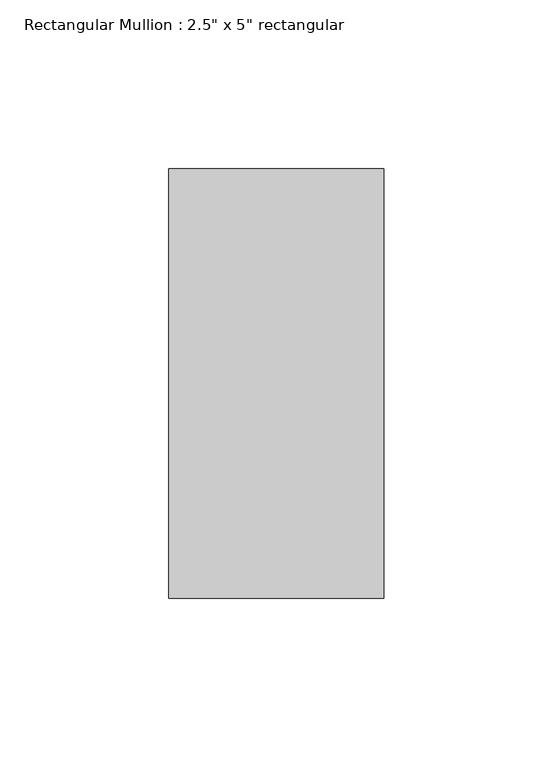
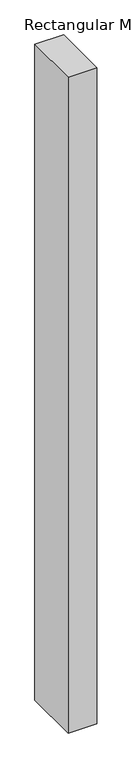
"""IFC4 building model written with IfcOpenShell, lengths in millimetres: member geometry."""

from ifc_helpers import new_model, si_unit, frame, origin, place, context, project, spatial, polyline, outline, extrude, source, transform, mapped, element, save


def member_9bd02798(model_context):
    return source(origin(), model_context, "Body", "SweptSolid", [
        extrude(outline(polyline([(0.0, 63.5), (0.0, -63.5), (-63.5, -63.5), (-63.5, 63.5), (0.0, 63.5)])), frame((0.0, 0.0, -1532.6819), z_axis=(0.0, 0.0, 1.0), x_axis=(1.0, 0.0, 0.0)), (0.0, 0.0, 1.0), 1532.6819),
    ])


if __name__ == "__main__":
    model = new_model("IFC4")
    model_context = context("Model", 3, world=origin())
    ifc_project = project(units=[si_unit("LENGTHUNIT", "METRE", prefix="MILLI")], contexts=[model_context])
    site = spatial("IfcSite", under=ifc_project)
    building = spatial("IfcBuilding", under=site)
    placement = place(None, origin())
    member_shape = member_9bd02798(model_context)
    element("IfcMember", 1, ObjectType="Rectangular Mullion : 2.5\" x 5\" rectangular", at=placement, inside=building, context=model_context, shape_type="MappedRepresentation", body=[
        mapped(member_shape, transform((0.0, 0.0, 0.0), x_axis=(1.0, 0.0, 0.0), y_axis=(0.0, 1.0, 0.0), z_axis=(0.0, 0.0, 1.0))),
    ])
    save(model, "model.ifc")

# Revit data of these elements
# Type "Rectangular Mullion : 2.5\" x 5\" rectangular"
#   built-in parameter 1007304 = 0.416667 (stored number, unit not read)
#   built-in parameter 1007301 = 0.104167 (stored number, unit not read)
#   built-in parameter 1007300 = 0.104167 (stored number, unit not read)
# Element 1 (IfcMember, "Rectangular Mullion : 2.5\" x 5\" rectangular")
#   Materials on its faces: "Aluminum"
# Materials
#   "Aluminum": class "Metal", colour RGB 247 247 247, transparency 0, Description = "Aluminum 6061", Cost = 0
